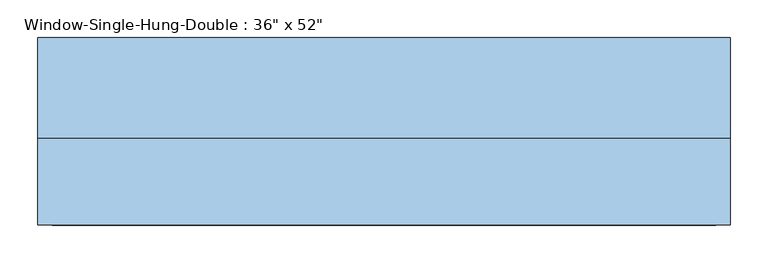
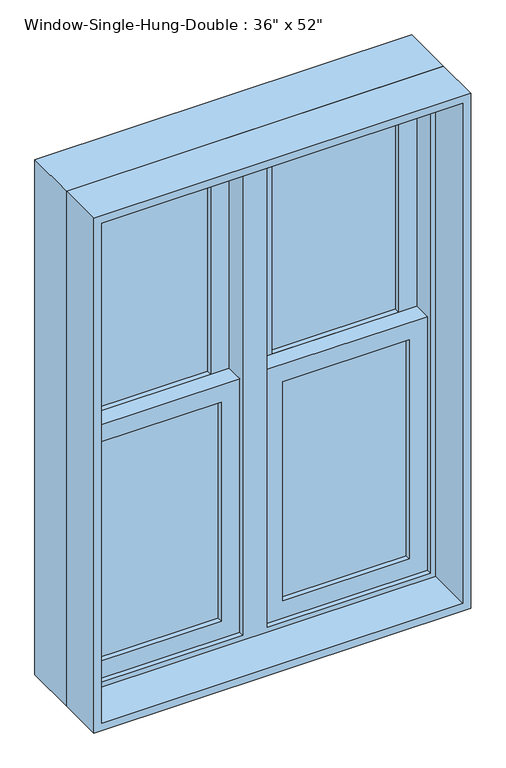
"""IFC4 building model written with IfcOpenShell, lengths in millimetres: window geometry."""

from ifc_helpers import new_model, si_unit, frame, origin, place, context, project, spatial, polyline, outline, extrude, source, transform, mapped, element, save


def window_45970670(model_context):
    return source(origin(), model_context, "Body", "SweptSolid", [
        extrude(outline(polyline([(2235.2, 457.2), (2235.2, -457.2), (914.4, -457.2), (914.4, 457.2), (2235.2, 457.2)]), holes=[polyline([(2216.15, 438.15), (933.45, 438.15), (933.45, -438.15), (2216.15, -438.15), (2216.15, 438.15)])]), frame((0.0, -114.3, 0.0), z_axis=(0.0, 1.0, 0.0), x_axis=(0.0, 0.0, 1.0)), (0.0, 0.0, 1.0), 114.3),
        extrude(outline(polyline([(2203.45, 30.1625), (1552.575, 30.1625), (1552.575, 425.45), (2203.45, 425.45), (2203.45, 30.1625)]), holes=[polyline([(2159.0, 381.0), (1597.025, 381.0), (1597.025, 74.6125), (2159.0, 74.6125), (2159.0, 381.0)])]), frame((0.0, 57.15, 0.0), z_axis=(0.0, 1.0, 0.0), x_axis=(0.0, 0.0, 1.0)), (0.0, 0.0, 1.0), 44.45),
        extrude(outline(polyline([(1597.025, 30.1625), (946.15, 30.1625), (946.15, 425.45), (1597.025, 425.45), (1597.025, 30.1625)]), holes=[polyline([(1552.575, 381.0), (990.6, 381.0), (990.6, 74.6125), (1552.575, 74.6125), (1552.575, 381.0)])]), frame((0.0, 12.7, 0.0), z_axis=(0.0, 1.0, 0.0), x_axis=(0.0, 0.0, 1.0)), (0.0, 0.0, 1.0), 44.45),
        extrude(outline(polyline([(381.0, 88.9), (381.0, 82.55), (74.6125, 82.55), (74.6125, 88.9), (381.0, 88.9)])), frame((0.0, 0.0, 1597.025), z_axis=(0.0, 0.0, 1.0), x_axis=(1.0, 0.0, 0.0)), (0.0, 0.0, 1.0), 561.975),
        extrude(outline(polyline([(74.6125, 76.2), (381.0, 76.2), (381.0, 69.85), (74.6125, 69.85), (74.6125, 76.2)])), frame((0.0, 0.0, 1597.025), z_axis=(0.0, 0.0, 1.0), x_axis=(1.0, 0.0, 0.0)), (0.0, 0.0, 1.0), 561.975),
        extrude(outline(polyline([(381.0, 44.45), (381.0, 38.1), (74.6125, 38.1), (74.6125, 44.45), (381.0, 44.45)])), frame((0.0, 0.0, 990.6), z_axis=(0.0, 0.0, 1.0), x_axis=(1.0, 0.0, 0.0)), (0.0, 0.0, 1.0), 561.975),
        extrude(outline(polyline([(74.6125, 31.75), (381.0, 31.75), (381.0, 25.4), (74.6125, 25.4), (74.6125, 31.75)])), frame((0.0, 0.0, 990.6), z_axis=(0.0, 0.0, 1.0), x_axis=(1.0, 0.0, 0.0)), (0.0, 0.0, 1.0), 561.975),
        extrude(outline(polyline([(2203.45, -425.45), (1552.575, -425.45), (1552.575, -30.1625), (2203.45, -30.1625), (2203.45, -425.45)]), holes=[polyline([(2159.0, -74.6125), (1597.025, -74.6125), (1597.025, -381.0), (2159.0, -381.0), (2159.0, -74.6125)])]), frame((0.0, 57.15, 0.0), z_axis=(0.0, 1.0, 0.0), x_axis=(0.0, 0.0, 1.0)), (0.0, 0.0, 1.0), 44.45),
        extrude(outline(polyline([(1597.025, -425.45), (946.15, -425.45), (946.15, -30.1625), (1597.025, -30.1625), (1597.025, -425.45)]), holes=[polyline([(1552.575, -74.6125), (990.6, -74.6125), (990.6, -381.0), (1552.575, -381.0), (1552.575, -74.6125)])]), frame((0.0, 12.7, 0.0), z_axis=(0.0, 1.0, 0.0), x_axis=(0.0, 0.0, 1.0)), (0.0, 0.0, 1.0), 44.45),
        extrude(outline(polyline([(-381.0, 88.9), (-74.6125, 88.9), (-74.6125, 82.55), (-381.0, 82.55), (-381.0, 88.9)])), frame((0.0, 0.0, 1597.025), z_axis=(0.0, 0.0, 1.0), x_axis=(1.0, 0.0, 0.0)), (0.0, 0.0, 1.0), 561.975),
        extrude(outline(polyline([(-74.6125, 76.2), (-74.6125, 69.85), (-381.0, 69.85), (-381.0, 76.2), (-74.6125, 76.2)])), frame((0.0, 0.0, 1597.025), z_axis=(0.0, 0.0, 1.0), x_axis=(1.0, 0.0, 0.0)), (0.0, 0.0, 1.0), 561.975),
        extrude(outline(polyline([(-381.0, 44.45), (-74.6125, 44.45), (-74.6125, 38.1), (-381.0, 38.1), (-381.0, 44.45)])), frame((0.0, 0.0, 990.6), z_axis=(0.0, 0.0, 1.0), x_axis=(1.0, 0.0, 0.0)), (0.0, 0.0, 1.0), 561.975),
        extrude(outline(polyline([(-74.6125, 31.75), (-74.6125, 25.4), (-381.0, 25.4), (-381.0, 31.75), (-74.6125, 31.75)])), frame((0.0, 0.0, 990.6), z_axis=(0.0, 0.0, 1.0), x_axis=(1.0, 0.0, 0.0)), (0.0, 0.0, 1.0), 561.975),
        extrude(outline(polyline([(2235.2, 457.2), (2235.2, -457.2), (914.4, -457.2), (914.4, 457.2), (2235.2, 457.2)]), holes=[polyline([(946.15, -425.45), (2203.45, -425.45), (2203.45, -30.1625), (946.15, -30.1625), (946.15, -425.45)]), polyline([(946.15, 425.45), (946.15, 30.1625), (2203.45, 30.1625), (2203.45, 425.45), (946.15, 425.45)])]), frame((0.0, 0.0, 0.0), z_axis=(0.0, 1.0, 0.0), x_axis=(0.0, 0.0, 1.0)), (0.0, 0.0, 1.0), 133.35),
    ])


if __name__ == "__main__":
    model = new_model("IFC4")
    model_context = context("Model", 3, world=origin())
    ifc_project = project(units=[si_unit("LENGTHUNIT", "METRE", prefix="MILLI")], contexts=[model_context])
    site = spatial("IfcSite", under=ifc_project)
    building = spatial("IfcBuilding", under=site)
    placement = place(None, origin())
    window_shape = window_45970670(model_context)
    element("IfcWindow", 1, ObjectType="Window-Single-Hung-Double : 36\" x 52\"", at=placement, inside=building, context=model_context, shape_type="MappedRepresentation", body=[
        mapped(window_shape, transform((0.0, 0.0, 0.0), x_axis=(1.0, 0.0, 0.0), y_axis=(0.0, 1.0, 0.0), z_axis=(0.0, 0.0, 1.0))),
    ])
    save(model, "model.ifc")

# Revit data of these elements
# Type "Window-Single-Hung-Double : 36\" x 52\""
#   Type Mark = "27"
#   Fire Rating = "0.5h"
#   Construction Type Id = "DG-DR"
#   Assembly Code = "B2020100"
#   Analytic Construction = "Double glazing - domestic"
#   Wall Thickness [instance default] = 0' - 6"
#   Window Inset [instance default] = 0' - 0"
#   Visual Light Transmittance = 0.81
#   Thermal Resistance (R) = 1.8146 (h·ft²·°F)/BTU
#   Solar Heat Gain Coefficient = 0.76
#   Muntin Width = 1' - 0 1/16"
#   Muntin Height = 1' - 10 1/8"
#   Interior Wall Closure [instance default] = 0' - 1 1/2"
#   Rough Width = 3' - 0 1/2"
#   Rough Height = 4' - 4 1/2"
#   Frame Extension [instance default] = 0' - 1 1/4"
#   Exterior Wall Closure [instance default] = 0' - 0 1/2"
#   Extension Jamb [instance default] = 0' - 1 1/2"
#   Heat Transfer Coefficient (U) = 0.5511 BTU/(h·ft²·°F)
#   Height = 4' - 4"
#   Width = 3' - 0"
#   Top Muntin Visibility = yes
#   Indicator Visibility [instance default] = yes
#   Extension Jamb Visibility [instance default] = yes
#   Interior Trim Visibility [instance default] = yes
#   Exterior Trim Visibility [instance default] = yes
#   Define Thermal Properties by = 1
#   Bottom Muntin Visibility = yes
#   Muntin Pattern = Muntin Pattern_2x2 : Muntin Pattern_2x2
#   Interior Trim = Trim-Window-Interior-Flat : Picture Frame
#   Interior Trim Material = Wood - Stained
#   Exterior Trim Material = Clad - White
#   Exterior Trim = Trim-Window-Exterior-Flat : with Sill
#   Glass Panel Material = Glass
#   Exterior Frame Material = Clad - White
#   Interior Frame Material = Wood - Stained
#   Wall Closure = (empty or 0)
# Element 1 (IfcWindow, "Window-Single-Hung-Double : 36\" x 52\"")
#   Wall Thickness = 0' - 9"
#   Extension Jamb = 0' - 4 1/2"
#   Materials on its faces: "Wood - Stained", "Glass", "Clad - White"
# Materials
#   "Wood - Stained": class "Wood", colour RGB 224 178 126, transparency 0, Cost = 0
#   "Clad - White": class "Wood", colour RGB 242 242 238, transparency 0, Cost = 0
#   "Glass": class "Glass", colour RGB 0 128 192, transparency 0.75, Description = "Soda Lime Glass", Cost = 0
